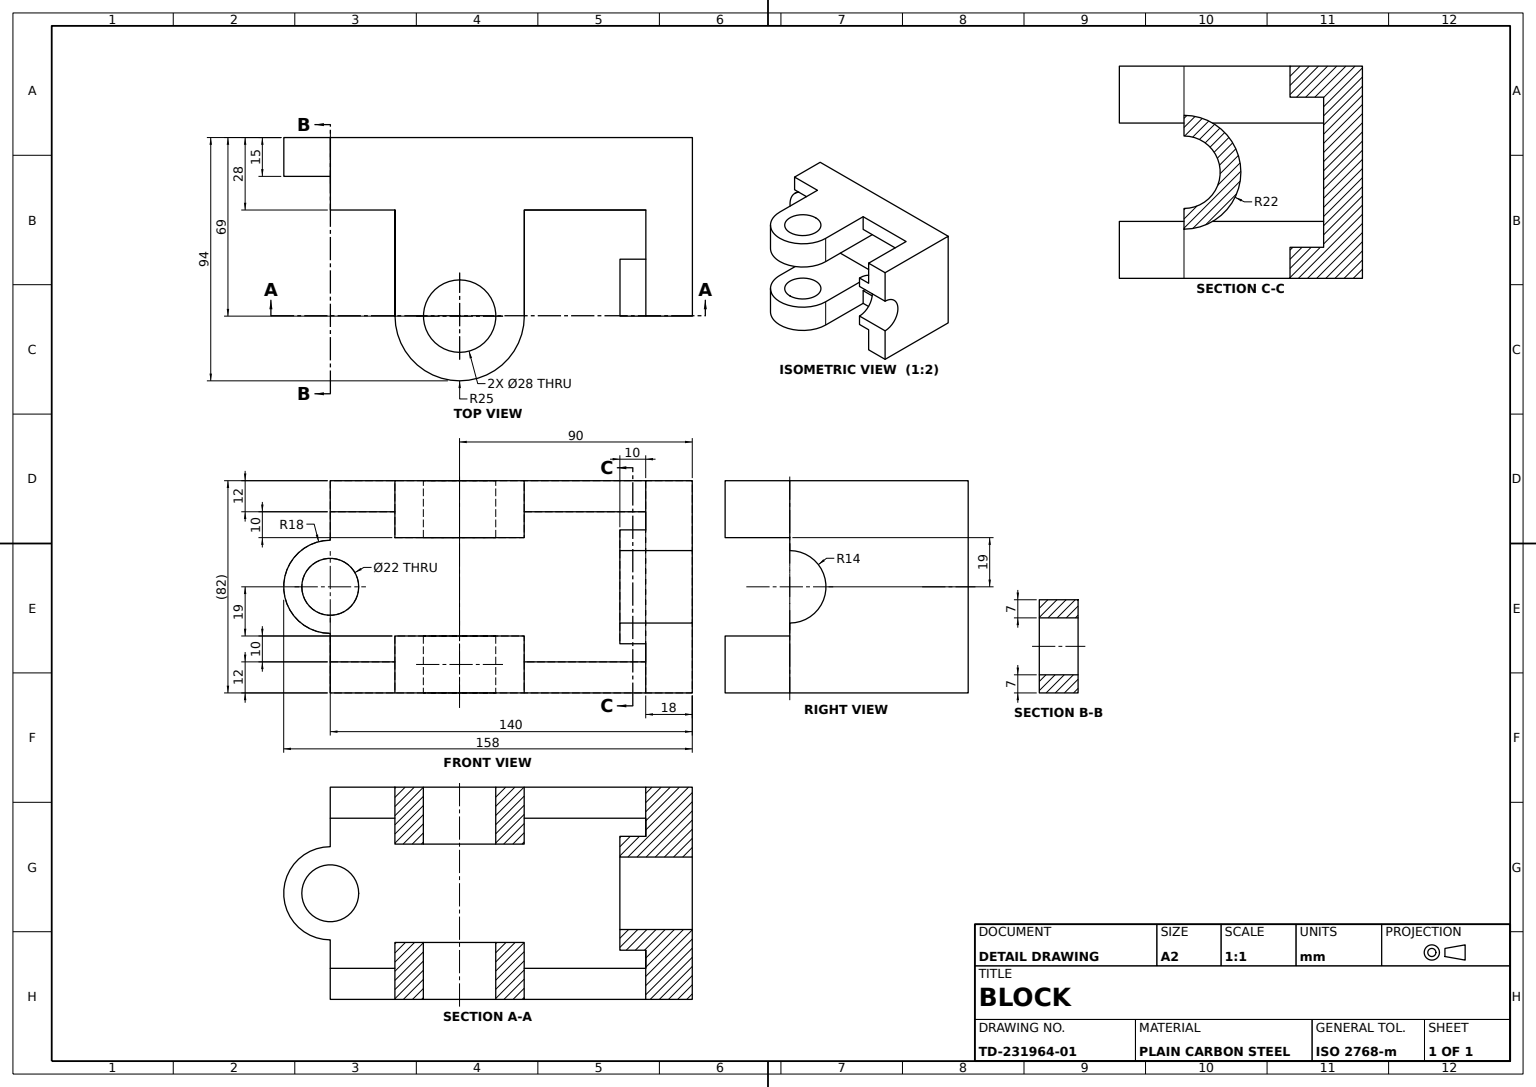
SolidWorks part; units mm, degrees
material "Plain Carbon Steel"
ref_plane "Front Plane" through (0, 0, 0) normal (0, 0, 1) x (1, 0, 0)
ref_plane "Top Plane" through (0, 0, 0) normal (0, 1, 0) x (1, 0, 0)
ref_plane "Right Plane" through (0, 0, 0) normal (1, 0, 0) x (0, 0, -1)
sketch "Base Plate Sketch" plane through (0, 0, 0) normal (0, 0, 1) x (1, 0, 0)
  line L0 (0, 0) -> (140, 0)
  line L1 (140, 0) -> (140, 82)
  line L2 (140, 82) -> (0, 82)
  line L3 (0, 82) -> (0, 0)
  dimension "D1" = 140
  dimension "D2" = 82
extrude "Base Plate" add sketch "Base Plate Sketch" along normal blind 15
sketch "Back Wall Sketch" plane through (140, 0, 0) normal (1, 0, 0) x (0, 0, -1)
  line L0 (-15, 82) -> (-69, 82)
  line L1 (-69, 82) -> (-69, 0)
  line L2 (-69, 0) -> (-15, 0)
  line L3 (-15, 0) -> (-15, 82) construction
  line L4 (-15, 0) -> (-15, 82)
  line L5 (0, 0) -> (0, 82) construction
  dimension "D1" = 69
extrude "Back Wall" add sketch "Back Wall Sketch" against normal blind 18
sketch "Rear Half Boss Sketch" plane through (122, 0, 0) normal (-1, 0, 0) x (0, 0, 1)
  line L0 (69, 82) -> (69, 0) construction
  line L1 (69, 63) -> (69, 19)
  arc A0 (69, 63) -> (69, 19) centre (69, 41) ccw
  dimension "D1" = 44
  dimension "D2" = 22
extrude "Rear Half Boss" add sketch "Rear Half Boss Sketch" along normal blind 10
sketch "Rear Half-Round Cut Sketch" plane through (112, 0, 0) normal (-1, 0, 0) x (0, 0, 1)
  line L0 (69, 19) -> (69, 63) construction
  line L1 (69, 55) -> (69, 27)
  arc A0 (69, 55) -> (69, 27) centre (69, 41) ccw
  dimension "D1" = 28
  dimension "D2" = 14
extrude "Rear Half-Round Cut" cut sketch "Rear Half-Round Cut Sketch" against normal blind 28
sketch "Lower Lug Sketch" plane through (0, 0, 0) normal (0, -1, 0) x (1, 0, 0)
  line L1 (0, 15) -> (122, 15) construction
  line L2 (75, 69) -> (75, 15)
  line L3 (25, 69) -> (25, 15)
  line L4 (75, 15) -> (25, 15)
  line L5 (140, 69) -> (140, 0) construction
  line L6 (0, 0) -> (140, 0) construction
  arc A0 (75, 69) -> (25, 69) centre (50, 69) ccw
  dimension "D1" = 50
  dimension "D2" = 25
  dimension "D3" = 90
  dimension "D4" = 69
extrude "Lower Lug" add sketch "Lower Lug Sketch" against normal blind 22
sketch "Spacer Block 1 Sketch" plane through (0, 0, 0) normal (0, -1, 0) x (1, 0, 0)
  line L0 (122, 15) -> (122, 28)
  line L1 (122, 69) -> (122, 15) construction
  line L2 (122, 28) -> (75, 28)
  line L3 (75, 15) -> (75, 69) construction
  line L4 (75, 28) -> (75, 15)
  line L5 (75, 15) -> (122, 15)
  line L7 (0, 0) -> (140, 0) construction
  dimension "D1" = 28
extrude "Spacer Block 1" add sketch "Spacer Block 1 Sketch" against normal blind 12
sketch "Spacer Block 2 Sketch" plane through (0, 0, 0) normal (0, -1, 0) x (1, 0, 0)
  line L0 (25, 15) -> (25, 28)
  line L1 (25, 69) -> (25, 15) construction
  line L2 (25, 28) -> (0, 28)
  line L3 (0, 28) -> (0, 15)
  line L4 (0, 15) -> (25, 15)
  dimension "D1" = 41
extrude "Spacer Block 2" add sketch "Spacer Block 2 Sketch" against normal blind 12
sketch "Spacer Block 3 Sketch" plane through (0, 82, 0) normal (0, 1, 0) x (1, 0, 0)
  line L0 (122, -15) -> (122, -28)
  line L1 (122, -28) -> (75, -28)
  line L2 (75, -28) -> (75, -15)
  line L3 (75, -15) -> (122, -15)
extrude "Spacer Block 3" add sketch "Spacer Block 3 Sketch" against normal blind 12
sketch "Upper Lug Sketch" plane through (0, 82, 0) normal (0, 1, 0) x (1, 0, 0)
  line L0 (25, -15) -> (75, -15)
  line L1 (75, -15) -> (75, -69)
  line L3 (25, -69) -> (25, -15)
  arc A0 (25, -69) -> (75, -69) centre (50, -69) ccw
  dimension "D1" = 50
extrude "Upper Lug" add sketch "Upper Lug Sketch" against normal blind 22
sketch "Spacer Block 4 Sketch" plane through (0, 82, 0) normal (0, 1, 0) x (1, 0, 0)
  line L0 (0, -15) -> (25, -15)
  line L1 (25, -15) -> (25, -28)
  line L2 (25, -28) -> (0, -28) construction
  line L3 (25, -15) -> (25, -28) construction
  line L4 (25, -28) -> (0, -28)
  line L5 (0, -28) -> (0, -15)
extrude "Spacer Block 4" add sketch "Spacer Block 4 Sketch" against normal blind 12
sketch "Side Half Boss Sketch" plane through (0, 0, 15) normal (0, 0, 1) x (1, 0, 0)
  line L0 (0, 70) -> (0, 12) construction
  line L1 (0, 59) -> (0, 23)
  arc A0 (0, 59) -> (0, 23) centre (0, 41) ccw
  dimension "D1" = 36
  dimension "D2" = 18
extrude "Side Half Boss" add sketch "Side Half Boss Sketch" against normal blind 15
sketch "Side Bore Sketch" plane through (0, 0, 15) normal (0, 0, 1) x (1, 0, 0)
  circle A0 centre (0, 41) radius 11
  dimension "D1" = 22
  dimension "D2" = 22
extrude "Side Bore Ø22" cut sketch "Side Bore Sketch" against normal blind 15
sketch "Upper Pin Hole Sketch" plane through (0, 82, 0) normal (0, 1, 0) x (1, 0, 0)
  circle A0 centre (50, -69) radius 14
  dimension "D1" = 28
  dimension "D2" = 28
extrude "Upper Lug Pin Hole Ø28" cut sketch "Upper Pin Hole Sketch" against normal blind 22
sketch "Lower Pin Hole Sketch" plane through (0, 0, 0) normal (0, -1, 0) x (1, 0, 0)
  circle A0 centre (50, 69) radius 14
  dimension "D1" = 28
  dimension "D2" = 28
extrude "Lower Lug Pin Hole Ø28" cut sketch "Lower Pin Hole Sketch" against normal blind 22
